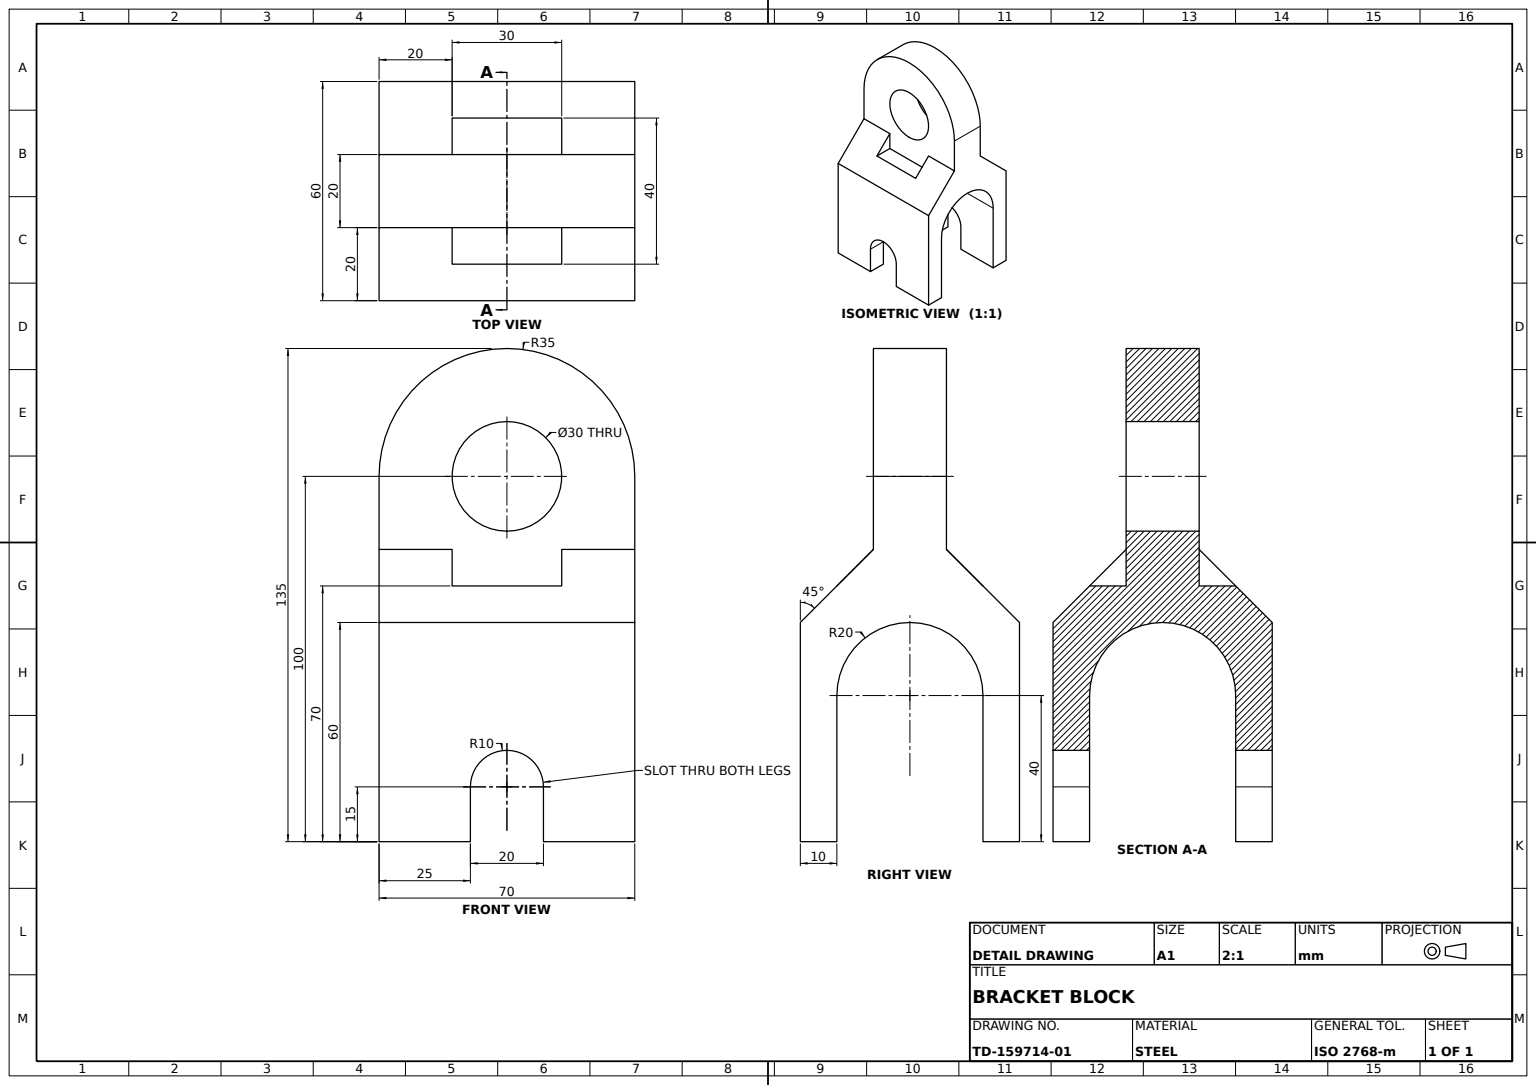
SolidWorks part; units mm, degrees
material "Plain Carbon Steel"
ref_plane "Front Plane" through (0, 0, 0) normal (0, 0, 1) x (1, 0, 0)
ref_plane "Top Plane" through (0, 0, 0) normal (0, 1, 0) x (1, 0, 0)
ref_plane "Right Plane" through (0, 0, 0) normal (1, 0, 0) x (0, 0, -1)
sketch "Arched Base Profile Sketch" plane through (0, 0, 0) normal (1, 0, 0) x (0, 0, -1)
  line L1 (-30, 0) -> (-10, 20)
  line L3 (-30, 0) -> (-30, -60)
  line L5 (-30, -60) -> (-20, -60)
  line L6 (30, 0) -> (30, -60)
  line L8 (10, 20) -> (30, 0)
  line L9 (-20, -60) -> (-20, -20)
  line L10 (20, -20) -> (20, -60)
  line L11 (20, -60) -> (30, -60)
  line L14 (-10, 20) -> (-10, 40)
  line L15 (-10, 40) -> (10, 40)
  line L16 (10, 20) -> (10, 40)
  arc A0 (-20, -20) -> (20, -20) centre (0, -20) cw
  point P5 (0, 40)
  point P12 (0, 0)
  dimension "D8" = 20
  dimension "D1" = 60
  dimension "D2" = 60
  dimension "D3" = 20
  dimension "D4" = 20
  dimension "D5" = 20
  dimension "D6" = 10
  dimension "D7" = 40
extrude "Arched Base Block" add sketch "Arched Base Profile Sketch" along normal mid plane 70
sketch "Hinge Ear Sketch" plane through (0, 0, -10) normal (0, 0, -1) x (-1, 0, 0)
  line L0 (-35, 40) -> (35, 40)
  arc A0 (-35, 40) -> (35, 40) centre (0, 40) cw
  dimension "D1" = 35
extrude "Hinge Ear" add sketch "Hinge Ear Sketch" against normal blind 20
sketch "Hinge Bore Sketch" plane through (0, 0, -10) normal (0, 0, -1) x (-1, 0, 0)
  line L0 (-10, -45) -> (-10, -60)
  line L1 (10, -45) -> (10, -60)
  line L2 (-35, -60) -> (35, -60) construction
  line L3 (10, -60) -> (-10, -60)
  circle A0 centre (0, 40) radius 15
  arc A2 (35, 40) -> (-35, 40) centre (0, 40) ccw construction
  arc A3 (10, -45) -> (-10, -45) centre (0, -45) ccw
  dimension "D1" = 30
  dimension "D2" = 20
  dimension "D3" = 15
extrude "Hinge Bore" cut sketch "Hinge Bore Sketch" against normal through all both and the other way through all
sketch "Ear Root Notch Sketch" plane through (0, 0, 0) normal (0, 1, 0) x (1, 0, 0)
  line L0 (35, 10) -> (-35, 10) construction
  line L1 (-15, 10) -> (15, 10)
  line L2 (-15, 10) -> (-15, 20)
  line L3 (-15, 20) -> (15, 20)
  line L4 (15, 10) -> (15, 20)
  line L5 (35, 30) -> (35, 10) construction
  point P6 (0, 20)
  dimension "D1" = 10
  dimension "D2" = 20
extrude "Ear Root Notch" cut sketch "Ear Root Notch Sketch" against normal blind 10 from offset 20
mirror "Ear Root Notch Mirror" about plane through (0, 0, 0) normal (0, 0, 1) of "Ear Root Notch"
